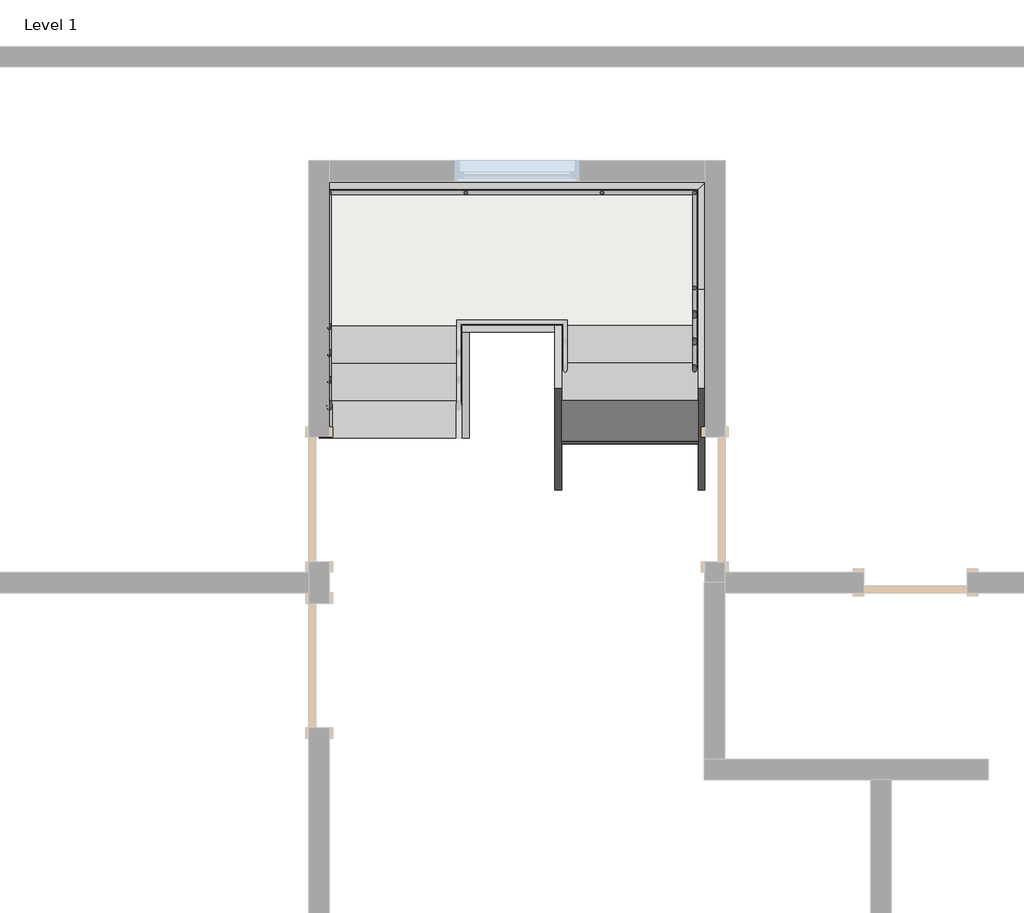
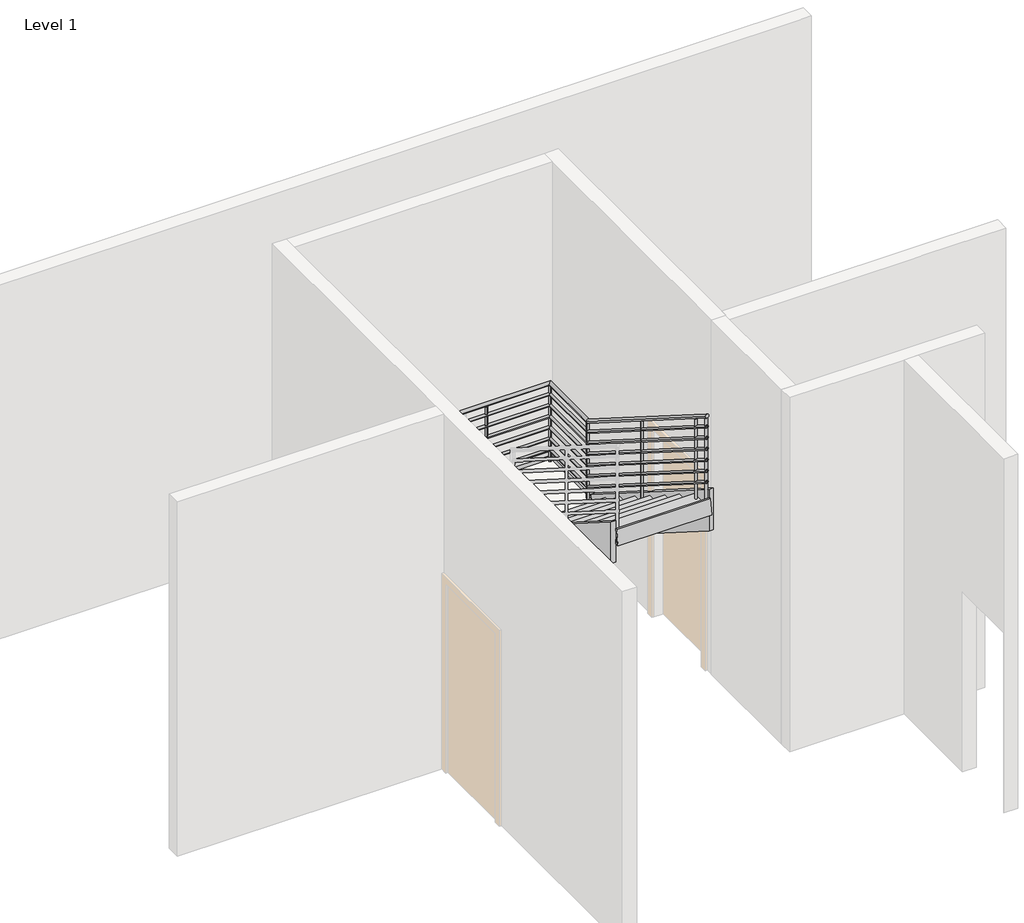
# One storey, part 3 of 3: 8 members, 2 stair flights, 1 railing, 1 slab.
"""IFC4 building model written with IfcOpenShell, lengths in millimetres."""

from ifc_helpers import new_model, si_unit, point, frame, frame_2d, origin, place, context, project, spatial, polyline, circle_curve, ellipse_curve, trimmed, segment, composite_curve, outline, extrude, faceted_brep, transform, mapped, element, save
from ifc_brep_helpers import plane_surface, cylinder_surface, advanced_brep
from components import non_monolithic_landing_4bf2fde8, stair_flight_50mm_tread_25mm_nosing_13mm_riser_7e2cbec3, stair_flight_50mm_tread_25mm_nosing_13mm_riser_d224a7c8

model = new_model("IFC4")

# Units and contexts
model_context = context("Model", 3, world=origin())
ifc_project = project(units=[si_unit("LENGTHUNIT", "METRE", prefix="MILLI")], contexts=[model_context])

# Site, building, storey
site = spatial("IfcSite", under=ifc_project)
building = spatial("IfcBuilding", under=site)
storey = spatial("IfcBuildingStorey", under=building, Name="Level 1", Elevation=0.0)

# Members
placement = place(None, origin())
element("IfcMember", 1, ObjectType="Stringer - 50mm Width", at=placement, inside=storey, context=model_context, shape_type="SweptSolid", body=[
    extrude(outline(polyline([(8997.57664, 0.0), (8997.57664, 215.089535), (9832.4076435, 743.0459009), (9948.2767035, 343.0459009), (9405.8353728, 0.0), (8997.57664, 0.0)])), frame((-10647.1504953, 0.0, 0.0), z_axis=(1.0, 0.0, 0.0), x_axis=(0.0, 1.0, 0.0)), (0.0, 0.0, 1.0), 50.0),
])
element("IfcMember", 2, ObjectType="Stringer - 50mm Width", at=placement, inside=storey, context=model_context, shape_type="SweptSolid", body=[
    extrude(outline(polyline([(8997.57664, 0.0), (8997.57664, 215.089535), (9772.57664, 705.2081121), (9772.57664, 231.9312362), (9405.8353728, 0.0), (8997.57664, 0.0)])), frame((-9597.1247141, 0.0, 0.0), z_axis=(1.0, 0.0, 0.0), x_axis=(0.0, 1.0, 0.0)), (0.0, 0.0, 1.0), 50.0),
])
element("IfcMember", 3, ObjectType="Stringer - 50mm Width", at=placement, inside=storey, context=model_context, shape_type="SweptSolid", body=[
    extrude(outline(polyline([(10087.7456364, 743.0459009), (9971.8765764, 343.0459009), (7897.57664, 1654.8561374), (7897.57664, 2128.1330133), (10087.7456364, 743.0459009)])), frame((-7867.4883818, 0.0, 0.0), z_axis=(1.0, 0.0, 0.0), x_axis=(0.0, 1.0, 0.0)), (0.0, 0.0, 1.0), 50.0),
])
element("IfcMember", 4, ObjectType="Stringer - 50mm Width", at=placement, inside=storey, context=model_context, shape_type="SweptSolid", body=[
    extrude(outline(polyline([(9822.57664, 910.7417089), (9822.57664, 437.464833), (7897.57664, 1654.8561374), (7897.57664, 2128.1330133), (9822.57664, 910.7417089)])), frame((-8917.5141631, 0.0, 0.0), z_axis=(1.0, 0.0, 0.0), x_axis=(0.0, 1.0, 0.0)), (0.0, 0.0, 1.0), 50.0),
])
element("IfcMember", 5, ObjectType="Stringer - 50mm Width", at=placement, inside=storey, context=model_context, shape_type="Brep", body=[
    faceted_brep([(-7867.4883818, 10087.7456364, 743.0459009), (-7817.4883818, 10087.7456364, 743.0459009), (-7817.4883818, 10872.6024212, 743.0459009), (-7867.4883818, 10822.6024212, 743.0459009), (-7867.4883818, 9971.8765764, 343.0459009), (-7867.4883818, 10822.6024212, 343.0459009), (-7817.4883818, 9971.8765764, 343.0459009), (-7817.4883818, 10872.6024212, 343.0459009)], [[[0, 1, 2, 3]], [[4, 0, 3, 5]], [[6, 4, 5, 7]], [[1, 6, 7, 2]], [[1, 0, 4, 6]], [[2, 7, 5, 3]]]),
])
element("IfcMember", 6, ObjectType="Stringer - 50mm Width", at=placement, inside=storey, context=model_context, shape_type="SweptSolid", body=[
    extrude(outline(polyline([(-7817.4883818, 10872.6024212), (-7867.4883818, 10822.6024212), (-10597.1504953, 10822.6024212), (-10647.1504953, 10872.6024212), (-7817.4883818, 10872.6024212)])), frame((0.0, 0.0, 343.0459009), z_axis=(0.0, 0.0, 1.0), x_axis=(1.0, 0.0, 0.0)), (0.0, 0.0, 1.0), 400.0),
])
element("IfcMember", 7, ObjectType="Stringer - 50mm Width", at=placement, inside=storey, context=model_context, shape_type="Brep", body=[
    faceted_brep([(-10597.1504953, 10822.6024212, 743.0459009), (-10647.1504953, 10872.6024212, 743.0459009), (-10647.1504953, 9832.4076435, 743.0459009), (-10597.1504953, 9832.4076435, 743.0459009), (-10597.1504953, 10822.6024212, 343.0459009), (-10597.1504953, 9948.2767035, 343.0459009), (-10647.1504953, 10872.6024212, 343.0459009), (-10647.1504953, 9948.2767035, 343.0459009)], [[[0, 1, 2, 3]], [[4, 0, 3, 5]], [[6, 4, 5, 7]], [[1, 6, 7, 2]], [[1, 0, 4, 6]], [[2, 7, 5, 3]]]),
])
element("IfcMember", 8, ObjectType="Stringer - 50mm Width", at=placement, inside=storey, context=model_context, shape_type="SweptSolid", body=[
    extrude(outline(polyline([(-9597.1247141, 9772.57664), (-9597.1247141, 9822.57664), (-8917.5141631, 9822.57664), (-8917.5141631, 9772.57664), (-9597.1247141, 9772.57664)])), frame((0.0, 0.0, 343.0459009), z_axis=(0.0, 0.0, 1.0), x_axis=(1.0, 0.0, 0.0)), (0.0, 0.0, 1.0), 400.0),
])

# Railing
element("IfcRailing", 9, ObjectType="900mm Pipe", at=placement, inside=storey, context=model_context, shape_type="SolidModel", body=[
    advanced_brep(
    [(-10551.7504953, 8997.57664, 1050.2491997), (-10591.7504953, 8997.57664, 1050.2491997), (-10551.7504953, 9828.370093, 1575.6521739), (-10591.7504953, 9828.370093, 1575.6521739), (-10551.7504953, 10777.2024212, 1575.6521739), (-10591.7504953, 10817.2024212, 1575.6521739), (-7912.8883818, 10777.2024212, 1575.6521739), (-7872.8883818, 10817.2024212, 1575.6521739), (-7912.8883818, 10091.783187, 1575.6521739), (-7872.8883818, 10091.783187, 1575.6521739), (-7912.8883818, 7897.57664, 2963.2926779), (-7872.8883818, 7897.57664, 2963.2926779)],
    [
        (0, 1, ellipse_curve(frame((-10571.7504953, 8997.57664, 1050.2491997), z_axis=(0.0, -1.0, 0.0), x_axis=(0.0, 0.0, -1.0)), 23.6638438, 20.0)),
        (1, 0, ellipse_curve(frame((-10571.7504953, 8997.57664, 1050.2491997), z_axis=(0.0, -1.0, 0.0), x_axis=(0.0, 0.0, -1.0)), 23.6638438, 20.0)),
        (0, 2),
        (2, 3, ellipse_curve(frame((-10571.7504953, 9828.370093, 1575.6521739), z_axis=(0.0, -0.9605132043335082, -0.27823440531497284), x_axis=(0.0, 0.2782344053149736, -0.9605132043335078)), 20.822202, 20.0)),
        (3, 1),
        (3, 2, ellipse_curve(frame((-10571.7504953, 9828.370093, 1575.6521739), z_axis=(0.0, -0.9605132043335082, -0.27823440531497284), x_axis=(0.0, 0.2782344053149736, -0.9605132043335078)), 20.822202, 20.0)),
        (2, 4),
        (4, 5, ellipse_curve(frame((-10571.7504953, 10797.2024212, 1575.6521739), z_axis=(-0.7071067811865475, -0.7071067811865475, 0.0), x_axis=(0.7071067811865474, -0.7071067811865476, 0.0)), 28.2842712, 20.0)),
        (5, 3),
        (5, 4, ellipse_curve(frame((-10571.7504953, 10797.2024212, 1575.6521739), z_axis=(-0.7071067811865475, -0.7071067811865475, 0.0), x_axis=(0.7071067811865474, -0.7071067811865476, 0.0)), 28.2842712, 20.0)),
        (4, 6),
        (6, 7, ellipse_curve(frame((-7892.8883818, 10797.2024212, 1575.6521739), z_axis=(-0.7071067811865475, 0.7071067811865475, 0.0), x_axis=(-0.7071067811865476, -0.7071067811865474, 0.0)), 28.2842712, 20.0)),
        (7, 5),
        (7, 6, ellipse_curve(frame((-7892.8883818, 10797.2024212, 1575.6521739), z_axis=(-0.7071067811865475, 0.7071067811865475, 0.0), x_axis=(-0.7071067811865476, -0.7071067811865474, 0.0)), 28.2842712, 20.0)),
        (6, 8),
        (8, 9, ellipse_curve(frame((-7892.8883818, 10091.783187, 1575.6521739), z_axis=(0.0, 0.9605132043335072, -0.27823440531497556), x_axis=(0.0, 0.27823440531497606, 0.9605132043335073)), 20.822202, 20.0)),
        (9, 7),
        (9, 8, ellipse_curve(frame((-7892.8883818, 10091.783187, 1575.6521739), z_axis=(0.0, 0.9605132043335072, -0.27823440531497556), x_axis=(0.0, 0.27823440531497606, 0.9605132043335073)), 20.822202, 20.0)),
        (10, 11, ellipse_curve(frame((-7892.8883818, 7897.57664, 2963.2926779), z_axis=(0.0, -1.0, 0.0), x_axis=(0.0, 0.0, -1.0)), 23.6638438, 20.0)),
        (11, 10, ellipse_curve(frame((-7892.8883818, 7897.57664, 2963.2926779), z_axis=(0.0, -1.0, 0.0), x_axis=(0.0, 0.0, -1.0)), 23.6638438, 20.0)),
        (8, 10),
        (11, 9),
    ],
    [
        plane_surface(frame((-10571.7504953, 8997.57664, 1073.9130435), z_axis=(0.0, -1.0, 0.0), x_axis=(0.0, 0.0, 1.0))),
        cylinder_surface(frame((-10571.7504953, 9008.2665528, 1057.0096189), z_axis=(0.0, -0.8451712313980468, -0.5344956404098252), x_axis=(-1.0, 0.0, 0.0)), 20.0),
        cylinder_surface(frame((-10571.7504953, 9822.57664, 1575.6521739), z_axis=(0.0, -1.0, 0.0), x_axis=(-1.0, 0.0, 0.0)), 20.0),
        cylinder_surface(frame((-10571.7504953, 10797.2024212, 1575.6521739), z_axis=(-1.0, 0.0, 0.0), x_axis=(0.0, 1.0, 0.0)), 20.0),
        cylinder_surface(frame((-7892.8883818, 10797.2024212, 1575.6521739), z_axis=(0.0, 1.0, 0.0), x_axis=(1.0, 0.0, 0.0)), 20.0),
        plane_surface(frame((-7892.8883818, 7897.57664, 2986.9565217), z_axis=(0.0, -1.0, 0.0), x_axis=(0.0, 0.0, -1.0))),
        cylinder_surface(frame((-7892.8883818, 10086.8867272, 1578.7487493), z_axis=(0.0, 0.8451712313980437, -0.5344956404098301), x_axis=(1.0, 0.0, 0.0)), 20.0),
    ],
    [
        (0, [[1, 2]]),
        (1, [[-1, 3, 4, 5]]),
        (1, [[-2, -5, 6, -3]]),
        (2, [[-4, 7, 8, 9]]),
        (2, [[-6, -9, 10, -7]]),
        (3, [[-8, 11, 12, 13]]),
        (3, [[-10, -13, 14, -11]]),
        (4, [[-12, 15, 16, 17]]),
        (4, [[-14, -17, 18, -15]]),
        (5, [[19, 20]]),
        (6, [[-16, 21, -20, 22]]),
        (6, [[-18, -22, -19, -21]]),
    ],
),
    advanced_brep(
    [(-10556.7504953, 8997.57664, 931.1651606), (-10586.7504953, 8997.57664, 931.1651606), (-10556.7504953, 9826.9217297, 1455.6521739), (-10586.7504953, 9826.9217297, 1455.6521739), (-10556.7504953, 10782.2024212, 1455.6521739), (-10586.7504953, 10812.2024212, 1455.6521739), (-7907.8883818, 10782.2024212, 1455.6521739), (-7877.8883818, 10812.2024212, 1455.6521739), (-7907.8883818, 10093.2315502, 1455.6521739), (-7877.8883818, 10093.2315502, 1455.6521739), (-7907.8883818, 7897.57664, 2844.2086389), (-7877.8883818, 7897.57664, 2844.2086389)],
    [
        (0, 1, ellipse_curve(frame((-10571.7504953, 8997.57664, 931.1651606), z_axis=(0.0, -1.0, 0.0), x_axis=(0.0, 0.0, -1.0)), 17.7478828, 15.0)),
        (1, 0, ellipse_curve(frame((-10571.7504953, 8997.57664, 931.1651606), z_axis=(0.0, -1.0, 0.0), x_axis=(0.0, 0.0, -1.0)), 17.7478828, 15.0)),
        (0, 2),
        (2, 3, ellipse_curve(frame((-10571.7504953, 9826.9217297, 1455.6521739), z_axis=(0.0, -0.9605132043335081, -0.2782344053149726), x_axis=(0.0, 0.27823440531497207, -0.9605132043335083)), 15.6166515, 15.0)),
        (3, 1),
        (3, 2, ellipse_curve(frame((-10571.7504953, 9826.9217297, 1455.6521739), z_axis=(0.0, -0.9605132043335081, -0.2782344053149726), x_axis=(0.0, 0.27823440531497207, -0.9605132043335083)), 15.6166515, 15.0)),
        (2, 4),
        (4, 5, ellipse_curve(frame((-10571.7504953, 10797.2024212, 1455.6521739), z_axis=(-0.7071067811865475, -0.7071067811865475, 0.0), x_axis=(0.7071067811865474, -0.7071067811865476, 0.0)), 21.2132034, 15.0)),
        (5, 3),
        (5, 4, ellipse_curve(frame((-10571.7504953, 10797.2024212, 1455.6521739), z_axis=(-0.7071067811865475, -0.7071067811865475, 0.0), x_axis=(0.7071067811865474, -0.7071067811865476, 0.0)), 21.2132034, 15.0)),
        (4, 6),
        (6, 7, ellipse_curve(frame((-7892.8883818, 10797.2024212, 1455.6521739), z_axis=(-0.7071067811865475, 0.7071067811865475, 0.0), x_axis=(-0.7071067811865476, -0.7071067811865474, 0.0)), 21.2132034, 15.0)),
        (7, 5),
        (7, 6, ellipse_curve(frame((-7892.8883818, 10797.2024212, 1455.6521739), z_axis=(-0.7071067811865475, 0.7071067811865475, 0.0), x_axis=(-0.7071067811865476, -0.7071067811865474, 0.0)), 21.2132034, 15.0)),
        (6, 8),
        (8, 9, ellipse_curve(frame((-7892.8883818, 10093.2315502, 1455.6521739), z_axis=(0.0, 0.9605132043335073, -0.27823440531497573), x_axis=(0.0, 0.27823440531497545, 0.9605132043335072)), 15.6166515, 15.0)),
        (9, 7),
        (9, 8, ellipse_curve(frame((-7892.8883818, 10093.2315502, 1455.6521739), z_axis=(0.0, 0.9605132043335073, -0.27823440531497573), x_axis=(0.0, 0.27823440531497545, 0.9605132043335072)), 15.6166515, 15.0)),
        (10, 11, ellipse_curve(frame((-7892.8883818, 7897.57664, 2844.2086389), z_axis=(0.0, -1.0, 0.0), x_axis=(0.0, 0.0, -1.0)), 17.7478828, 15.0)),
        (11, 10, ellipse_curve(frame((-7892.8883818, 7897.57664, 2844.2086389), z_axis=(0.0, -1.0, 0.0), x_axis=(0.0, 0.0, -1.0)), 17.7478828, 15.0)),
        (8, 10),
        (11, 9),
    ],
    [
        plane_surface(frame((-10571.7504953, 8997.57664, 948.9130435), z_axis=(0.0, -1.0, 0.0), x_axis=(0.0, 0.0, 1.0))),
        cylinder_surface(frame((-10571.7504953, 9005.5940746, 936.235475), z_axis=(0.0, -0.845171231398047, -0.534495640409825), x_axis=(-1.0, 0.0, 0.0)), 15.0),
        cylinder_surface(frame((-10571.7504953, 9822.57664, 1455.6521739), z_axis=(0.0, -1.0, 0.0), x_axis=(-1.0, 0.0, 0.0)), 15.0),
        cylinder_surface(frame((-10571.7504953, 10797.2024212, 1455.6521739), z_axis=(-1.0, 0.0, 0.0), x_axis=(0.0, 1.0, 0.0)), 15.0),
        cylinder_surface(frame((-7892.8883818, 10797.2024212, 1455.6521739), z_axis=(0.0, 1.0, 0.0), x_axis=(1.0, 0.0, 0.0)), 15.0),
        plane_surface(frame((-7892.8883818, 7897.57664, 2861.9565217), z_axis=(0.0, -1.0, 0.0), x_axis=(0.0, 0.0, -1.0))),
        cylinder_surface(frame((-7892.8883818, 10089.5592054, 1457.9746054), z_axis=(0.0, 0.8451712313980436, -0.5344956404098303), x_axis=(1.0, 0.0, 0.0)), 15.0),
    ],
    [
        (0, [[1, 2]]),
        (1, [[-1, 3, 4, 5]]),
        (1, [[-2, -5, 6, -3]]),
        (2, [[-4, 7, 8, 9]]),
        (2, [[-6, -9, 10, -7]]),
        (3, [[-8, 11, 12, 13]]),
        (3, [[-10, -13, 14, -11]]),
        (4, [[-12, 15, 16, 17]]),
        (4, [[-14, -17, 18, -15]]),
        (5, [[19, 20]]),
        (6, [[-16, 21, -20, 22]]),
        (6, [[-18, -22, -19, -21]]),
    ],
),
    advanced_brep(
    [(-10556.7504953, 8997.57664, 806.1651606), (-10586.7504953, 8997.57664, 806.1651606), (-10556.7504953, 9826.9217297, 1330.6521739), (-10586.7504953, 9826.9217297, 1330.6521739), (-10556.7504953, 10782.2024212, 1330.6521739), (-10586.7504953, 10812.2024212, 1330.6521739), (-7907.8883818, 10782.2024212, 1330.6521739), (-7877.8883818, 10812.2024212, 1330.6521739), (-7907.8883818, 10093.2315502, 1330.6521739), (-7877.8883818, 10093.2315502, 1330.6521739), (-7907.8883818, 7897.57664, 2719.2086389), (-7877.8883818, 7897.57664, 2719.2086389)],
    [
        (0, 1, ellipse_curve(frame((-10571.7504953, 8997.57664, 806.1651606), z_axis=(0.0, -1.0, 0.0), x_axis=(0.0, 0.0, -1.0)), 17.7478828, 15.0)),
        (1, 0, ellipse_curve(frame((-10571.7504953, 8997.57664, 806.1651606), z_axis=(0.0, -1.0, 0.0), x_axis=(0.0, 0.0, -1.0)), 17.7478828, 15.0)),
        (0, 2),
        (2, 3, ellipse_curve(frame((-10571.7504953, 9826.9217297, 1330.6521739), z_axis=(0.0, -0.9605132043335081, -0.2782344053149726), x_axis=(0.0, 0.27823440531497207, -0.9605132043335083)), 15.6166515, 15.0)),
        (3, 1),
        (3, 2, ellipse_curve(frame((-10571.7504953, 9826.9217297, 1330.6521739), z_axis=(0.0, -0.9605132043335081, -0.2782344053149726), x_axis=(0.0, 0.27823440531497207, -0.9605132043335083)), 15.6166515, 15.0)),
        (2, 4),
        (4, 5, ellipse_curve(frame((-10571.7504953, 10797.2024212, 1330.6521739), z_axis=(-0.7071067811865475, -0.7071067811865475, 0.0), x_axis=(0.7071067811865474, -0.7071067811865476, 0.0)), 21.2132034, 15.0)),
        (5, 3),
        (5, 4, ellipse_curve(frame((-10571.7504953, 10797.2024212, 1330.6521739), z_axis=(-0.7071067811865475, -0.7071067811865475, 0.0), x_axis=(0.7071067811865474, -0.7071067811865476, 0.0)), 21.2132034, 15.0)),
        (4, 6),
        (6, 7, ellipse_curve(frame((-7892.8883818, 10797.2024212, 1330.6521739), z_axis=(-0.7071067811865475, 0.7071067811865475, 0.0), x_axis=(-0.7071067811865476, -0.7071067811865474, 0.0)), 21.2132034, 15.0)),
        (7, 5),
        (7, 6, ellipse_curve(frame((-7892.8883818, 10797.2024212, 1330.6521739), z_axis=(-0.7071067811865475, 0.7071067811865475, 0.0), x_axis=(-0.7071067811865476, -0.7071067811865474, 0.0)), 21.2132034, 15.0)),
        (6, 8),
        (8, 9, ellipse_curve(frame((-7892.8883818, 10093.2315502, 1330.6521739), z_axis=(0.0, 0.9605132043335072, -0.2782344053149755), x_axis=(0.0, 0.27823440531497606, 0.9605132043335073)), 15.6166515, 15.0)),
        (9, 7),
        (9, 8, ellipse_curve(frame((-7892.8883818, 10093.2315502, 1330.6521739), z_axis=(0.0, 0.9605132043335072, -0.2782344053149755), x_axis=(0.0, 0.27823440531497606, 0.9605132043335073)), 15.6166515, 15.0)),
        (10, 11, ellipse_curve(frame((-7892.8883818, 7897.57664, 2719.2086389), z_axis=(0.0, -1.0, 0.0), x_axis=(0.0, 0.0, -1.0)), 17.7478828, 15.0)),
        (11, 10, ellipse_curve(frame((-7892.8883818, 7897.57664, 2719.2086389), z_axis=(0.0, -1.0, 0.0), x_axis=(0.0, 0.0, -1.0)), 17.7478828, 15.0)),
        (8, 10),
        (11, 9),
    ],
    [
        plane_surface(frame((-10571.7504953, 8997.57664, 823.9130435), z_axis=(0.0, -1.0, 0.0), x_axis=(0.0, 0.0, 1.0))),
        cylinder_surface(frame((-10571.7504953, 9005.5940746, 811.235475), z_axis=(0.0, -0.845171231398047, -0.534495640409825), x_axis=(-1.0, 0.0, 0.0)), 15.0),
        cylinder_surface(frame((-10571.7504953, 9822.57664, 1330.6521739), z_axis=(0.0, -1.0, 0.0), x_axis=(-1.0, 0.0, 0.0)), 15.0),
        cylinder_surface(frame((-10571.7504953, 10797.2024212, 1330.6521739), z_axis=(-1.0, 0.0, 0.0), x_axis=(0.0, 1.0, 0.0)), 15.0),
        cylinder_surface(frame((-7892.8883818, 10797.2024212, 1330.6521739), z_axis=(0.0, 1.0, 0.0), x_axis=(1.0, 0.0, 0.0)), 15.0),
        plane_surface(frame((-7892.8883818, 7897.57664, 2736.9565217), z_axis=(0.0, -1.0, 0.0), x_axis=(0.0, 0.0, -1.0))),
        cylinder_surface(frame((-7892.8883818, 10089.5592054, 1332.9746054), z_axis=(0.0, 0.8451712313980437, -0.5344956404098301), x_axis=(1.0, 0.0, 0.0)), 15.0),
    ],
    [
        (0, [[1, 2]]),
        (1, [[-1, 3, 4, 5]]),
        (1, [[-2, -5, 6, -3]]),
        (2, [[-4, 7, 8, 9]]),
        (2, [[-6, -9, 10, -7]]),
        (3, [[-8, 11, 12, 13]]),
        (3, [[-10, -13, 14, -11]]),
        (4, [[-12, 15, 16, 17]]),
        (4, [[-14, -17, 18, -15]]),
        (5, [[19, 20]]),
        (6, [[-16, 21, -20, 22]]),
        (6, [[-18, -22, -19, -21]]),
    ],
),
    advanced_brep(
    [(-10556.7504953, 8997.57664, 681.1651606), (-10586.7504953, 8997.57664, 681.1651606), (-10556.7504953, 9826.9217297, 1205.6521739), (-10586.7504953, 9826.9217297, 1205.6521739), (-10556.7504953, 10782.2024212, 1205.6521739), (-10586.7504953, 10812.2024212, 1205.6521739), (-7907.8883818, 10782.2024212, 1205.6521739), (-7877.8883818, 10812.2024212, 1205.6521739), (-7907.8883818, 10093.2315502, 1205.6521739), (-7877.8883818, 10093.2315502, 1205.6521739), (-7907.8883818, 7897.57664, 2594.2086389), (-7877.8883818, 7897.57664, 2594.2086389)],
    [
        (0, 1, ellipse_curve(frame((-10571.7504953, 8997.57664, 681.1651606), z_axis=(0.0, -1.0, 0.0), x_axis=(0.0, 0.0, -1.0)), 17.7478828, 15.0)),
        (1, 0, ellipse_curve(frame((-10571.7504953, 8997.57664, 681.1651606), z_axis=(0.0, -1.0, 0.0), x_axis=(0.0, 0.0, -1.0)), 17.7478828, 15.0)),
        (0, 2),
        (2, 3, ellipse_curve(frame((-10571.7504953, 9826.9217297, 1205.6521739), z_axis=(0.0, -0.9605132043335081, -0.2782344053149726), x_axis=(0.0, 0.27823440531497207, -0.9605132043335083)), 15.6166515, 15.0)),
        (3, 1),
        (3, 2, ellipse_curve(frame((-10571.7504953, 9826.9217297, 1205.6521739), z_axis=(0.0, -0.9605132043335081, -0.2782344053149726), x_axis=(0.0, 0.27823440531497207, -0.9605132043335083)), 15.6166515, 15.0)),
        (2, 4),
        (4, 5, ellipse_curve(frame((-10571.7504953, 10797.2024212, 1205.6521739), z_axis=(-0.7071067811865475, -0.7071067811865475, 0.0), x_axis=(0.7071067811865474, -0.7071067811865476, 0.0)), 21.2132034, 15.0)),
        (5, 3),
        (5, 4, ellipse_curve(frame((-10571.7504953, 10797.2024212, 1205.6521739), z_axis=(-0.7071067811865475, -0.7071067811865475, 0.0), x_axis=(0.7071067811865474, -0.7071067811865476, 0.0)), 21.2132034, 15.0)),
        (4, 6),
        (6, 7, ellipse_curve(frame((-7892.8883818, 10797.2024212, 1205.6521739), z_axis=(-0.7071067811865475, 0.7071067811865475, 0.0), x_axis=(-0.7071067811865476, -0.7071067811865474, 0.0)), 21.2132034, 15.0)),
        (7, 5),
        (7, 6, ellipse_curve(frame((-7892.8883818, 10797.2024212, 1205.6521739), z_axis=(-0.7071067811865475, 0.7071067811865475, 0.0), x_axis=(-0.7071067811865476, -0.7071067811865474, 0.0)), 21.2132034, 15.0)),
        (6, 8),
        (8, 9, ellipse_curve(frame((-7892.8883818, 10093.2315502, 1205.6521739), z_axis=(0.0, 0.9605132043335072, -0.2782344053149755), x_axis=(0.0, 0.27823440531497606, 0.9605132043335073)), 15.6166515, 15.0)),
        (9, 7),
        (9, 8, ellipse_curve(frame((-7892.8883818, 10093.2315502, 1205.6521739), z_axis=(0.0, 0.9605132043335072, -0.2782344053149755), x_axis=(0.0, 0.27823440531497606, 0.9605132043335073)), 15.6166515, 15.0)),
        (10, 11, ellipse_curve(frame((-7892.8883818, 7897.57664, 2594.2086389), z_axis=(0.0, -1.0, 0.0), x_axis=(0.0, 0.0, -1.0)), 17.7478828, 15.0)),
        (11, 10, ellipse_curve(frame((-7892.8883818, 7897.57664, 2594.2086389), z_axis=(0.0, -1.0, 0.0), x_axis=(0.0, 0.0, -1.0)), 17.7478828, 15.0)),
        (8, 10),
        (11, 9),
    ],
    [
        plane_surface(frame((-10571.7504953, 8997.57664, 698.9130435), z_axis=(0.0, -1.0, 0.0), x_axis=(0.0, 0.0, 1.0))),
        cylinder_surface(frame((-10571.7504953, 9005.5940746, 686.235475), z_axis=(0.0, -0.845171231398047, -0.534495640409825), x_axis=(-1.0, 0.0, 0.0)), 15.0),
        cylinder_surface(frame((-10571.7504953, 9822.57664, 1205.6521739), z_axis=(0.0, -1.0, 0.0), x_axis=(-1.0, 0.0, 0.0)), 15.0),
        cylinder_surface(frame((-10571.7504953, 10797.2024212, 1205.6521739), z_axis=(-1.0, 0.0, 0.0), x_axis=(0.0, 1.0, 0.0)), 15.0),
        cylinder_surface(frame((-7892.8883818, 10797.2024212, 1205.6521739), z_axis=(0.0, 1.0, 0.0), x_axis=(1.0, 0.0, 0.0)), 15.0),
        plane_surface(frame((-7892.8883818, 7897.57664, 2611.9565217), z_axis=(0.0, -1.0, 0.0), x_axis=(0.0, 0.0, -1.0))),
        cylinder_surface(frame((-7892.8883818, 10089.5592054, 1207.9746054), z_axis=(0.0, 0.8451712313980437, -0.5344956404098301), x_axis=(1.0, 0.0, 0.0)), 15.0),
    ],
    [
        (0, [[1, 2]]),
        (1, [[-1, 3, 4, 5]]),
        (1, [[-2, -5, 6, -3]]),
        (2, [[-4, 7, 8, 9]]),
        (2, [[-6, -9, 10, -7]]),
        (3, [[-8, 11, 12, 13]]),
        (3, [[-10, -13, 14, -11]]),
        (4, [[-12, 15, 16, 17]]),
        (4, [[-14, -17, 18, -15]]),
        (5, [[19, 20]]),
        (6, [[-16, 21, -20, 22]]),
        (6, [[-18, -22, -19, -21]]),
    ],
),
    advanced_brep(
    [(-10556.7504953, 8997.57664, 556.1651606), (-10586.7504953, 8997.57664, 556.1651606), (-10556.7504953, 9826.9217297, 1080.6521739), (-10586.7504953, 9826.9217297, 1080.6521739), (-10556.7504953, 10782.2024212, 1080.6521739), (-10586.7504953, 10812.2024212, 1080.6521739), (-7907.8883818, 10782.2024212, 1080.6521739), (-7877.8883818, 10812.2024212, 1080.6521739), (-7907.8883818, 10093.2315502, 1080.6521739), (-7877.8883818, 10093.2315502, 1080.6521739), (-7907.8883818, 7897.57664, 2469.2086389), (-7877.8883818, 7897.57664, 2469.2086389)],
    [
        (0, 1, ellipse_curve(frame((-10571.7504953, 8997.57664, 556.1651606), z_axis=(0.0, -1.0, 0.0), x_axis=(0.0, 0.0, -1.0)), 17.7478828, 15.0)),
        (1, 0, ellipse_curve(frame((-10571.7504953, 8997.57664, 556.1651606), z_axis=(0.0, -1.0, 0.0), x_axis=(0.0, 0.0, -1.0)), 17.7478828, 15.0)),
        (0, 2),
        (2, 3, ellipse_curve(frame((-10571.7504953, 9826.9217297, 1080.6521739), z_axis=(0.0, -0.9605132043335081, -0.27823440531497273), x_axis=(0.0, 0.2782344053149724, -0.9605132043335081)), 15.6166515, 15.0)),
        (3, 1),
        (3, 2, ellipse_curve(frame((-10571.7504953, 9826.9217297, 1080.6521739), z_axis=(0.0, -0.9605132043335081, -0.27823440531497273), x_axis=(0.0, 0.2782344053149724, -0.9605132043335081)), 15.6166515, 15.0)),
        (2, 4),
        (4, 5, ellipse_curve(frame((-10571.7504953, 10797.2024212, 1080.6521739), z_axis=(-0.7071067811865475, -0.7071067811865475, 0.0), x_axis=(0.7071067811865474, -0.7071067811865476, 0.0)), 21.2132034, 15.0)),
        (5, 3),
        (5, 4, ellipse_curve(frame((-10571.7504953, 10797.2024212, 1080.6521739), z_axis=(-0.7071067811865475, -0.7071067811865475, 0.0), x_axis=(0.7071067811865474, -0.7071067811865476, 0.0)), 21.2132034, 15.0)),
        (4, 6),
        (6, 7, ellipse_curve(frame((-7892.8883818, 10797.2024212, 1080.6521739), z_axis=(-0.7071067811865475, 0.7071067811865475, 0.0), x_axis=(-0.7071067811865476, -0.7071067811865474, 0.0)), 21.2132034, 15.0)),
        (7, 5),
        (7, 6, ellipse_curve(frame((-7892.8883818, 10797.2024212, 1080.6521739), z_axis=(-0.7071067811865475, 0.7071067811865475, 0.0), x_axis=(-0.7071067811865476, -0.7071067811865474, 0.0)), 21.2132034, 15.0)),
        (6, 8),
        (8, 9, ellipse_curve(frame((-7892.8883818, 10093.2315502, 1080.6521739), z_axis=(0.0, 0.9605132043335072, -0.2782344053149755), x_axis=(0.0, 0.27823440531497606, 0.9605132043335073)), 15.6166515, 15.0)),
        (9, 7),
        (9, 8, ellipse_curve(frame((-7892.8883818, 10093.2315502, 1080.6521739), z_axis=(0.0, 0.9605132043335072, -0.2782344053149755), x_axis=(0.0, 0.27823440531497606, 0.9605132043335073)), 15.6166515, 15.0)),
        (10, 11, ellipse_curve(frame((-7892.8883818, 7897.57664, 2469.2086389), z_axis=(0.0, -1.0, 0.0), x_axis=(0.0, 0.0, -1.0)), 17.7478828, 15.0)),
        (11, 10, ellipse_curve(frame((-7892.8883818, 7897.57664, 2469.2086389), z_axis=(0.0, -1.0, 0.0), x_axis=(0.0, 0.0, -1.0)), 17.7478828, 15.0)),
        (8, 10),
        (11, 9),
    ],
    [
        plane_surface(frame((-10571.7504953, 8997.57664, 573.9130435), z_axis=(0.0, -1.0, 0.0), x_axis=(0.0, 0.0, 1.0))),
        cylinder_surface(frame((-10571.7504953, 9005.5940746, 561.235475), z_axis=(0.0, -0.845171231398047, -0.5344956404098251), x_axis=(-1.0, 0.0, 0.0)), 15.0),
        cylinder_surface(frame((-10571.7504953, 9822.57664, 1080.6521739), z_axis=(0.0, -1.0, 0.0), x_axis=(-1.0, 0.0, 0.0)), 15.0),
        cylinder_surface(frame((-10571.7504953, 10797.2024212, 1080.6521739), z_axis=(-1.0, 0.0, 0.0), x_axis=(0.0, 1.0, 0.0)), 15.0),
        cylinder_surface(frame((-7892.8883818, 10797.2024212, 1080.6521739), z_axis=(0.0, 1.0, 0.0), x_axis=(1.0, 0.0, 0.0)), 15.0),
        plane_surface(frame((-7892.8883818, 7897.57664, 2486.9565217), z_axis=(0.0, -1.0, 0.0), x_axis=(0.0, 0.0, -1.0))),
        cylinder_surface(frame((-7892.8883818, 10089.5592054, 1082.9746054), z_axis=(0.0, 0.8451712313980437, -0.5344956404098301), x_axis=(1.0, 0.0, 0.0)), 15.0),
    ],
    [
        (0, [[1, 2]]),
        (1, [[-1, 3, 4, 5]]),
        (1, [[-2, -5, 6, -3]]),
        (2, [[-4, 7, 8, 9]]),
        (2, [[-6, -9, 10, -7]]),
        (3, [[-8, 11, 12, 13]]),
        (3, [[-10, -13, 14, -11]]),
        (4, [[-12, 15, 16, 17]]),
        (4, [[-14, -17, 18, -15]]),
        (5, [[19, 20]]),
        (6, [[-16, 21, -20, 22]]),
        (6, [[-18, -22, -19, -21]]),
    ],
),
    advanced_brep(
    [(-10556.7504953, 8997.57664, 431.1651606), (-10586.7504953, 8997.57664, 431.1651606), (-10556.7504953, 9826.9217297, 955.6521739), (-10586.7504953, 9826.9217297, 955.6521739), (-10556.7504953, 10782.2024212, 955.6521739), (-10586.7504953, 10812.2024212, 955.6521739), (-7907.8883818, 10782.2024212, 955.6521739), (-7877.8883818, 10812.2024212, 955.6521739), (-7907.8883818, 10093.2315502, 955.6521739), (-7877.8883818, 10093.2315502, 955.6521739), (-7907.8883818, 7897.57664, 2344.2086389), (-7877.8883818, 7897.57664, 2344.2086389)],
    [
        (0, 1, ellipse_curve(frame((-10571.7504953, 8997.57664, 431.1651606), z_axis=(0.0, -1.0, 0.0), x_axis=(0.0, 0.0, -1.0)), 17.7478828, 15.0)),
        (1, 0, ellipse_curve(frame((-10571.7504953, 8997.57664, 431.1651606), z_axis=(0.0, -1.0, 0.0), x_axis=(0.0, 0.0, -1.0)), 17.7478828, 15.0)),
        (0, 2),
        (2, 3, ellipse_curve(frame((-10571.7504953, 9826.9217297, 955.6521739), z_axis=(0.0, -0.9605132043335081, -0.27823440531497273), x_axis=(0.0, 0.2782344053149724, -0.9605132043335081)), 15.6166515, 15.0)),
        (3, 1),
        (3, 2, ellipse_curve(frame((-10571.7504953, 9826.9217297, 955.6521739), z_axis=(0.0, -0.9605132043335081, -0.27823440531497273), x_axis=(0.0, 0.2782344053149724, -0.9605132043335081)), 15.6166515, 15.0)),
        (2, 4),
        (4, 5, ellipse_curve(frame((-10571.7504953, 10797.2024212, 955.6521739), z_axis=(-0.7071067811865475, -0.7071067811865475, 0.0), x_axis=(0.7071067811865474, -0.7071067811865476, 0.0)), 21.2132034, 15.0)),
        (5, 3),
        (5, 4, ellipse_curve(frame((-10571.7504953, 10797.2024212, 955.6521739), z_axis=(-0.7071067811865475, -0.7071067811865475, 0.0), x_axis=(0.7071067811865474, -0.7071067811865476, 0.0)), 21.2132034, 15.0)),
        (4, 6),
        (6, 7, ellipse_curve(frame((-7892.8883818, 10797.2024212, 955.6521739), z_axis=(-0.7071067811865475, 0.7071067811865475, 0.0), x_axis=(-0.7071067811865476, -0.7071067811865474, 0.0)), 21.2132034, 15.0)),
        (7, 5),
        (7, 6, ellipse_curve(frame((-7892.8883818, 10797.2024212, 955.6521739), z_axis=(-0.7071067811865475, 0.7071067811865475, 0.0), x_axis=(-0.7071067811865476, -0.7071067811865474, 0.0)), 21.2132034, 15.0)),
        (6, 8),
        (8, 9, ellipse_curve(frame((-7892.8883818, 10093.2315502, 955.6521739), z_axis=(0.0, 0.9605132043335072, -0.2782344053149755), x_axis=(0.0, 0.27823440531497606, 0.9605132043335073)), 15.6166515, 15.0)),
        (9, 7),
        (9, 8, ellipse_curve(frame((-7892.8883818, 10093.2315502, 955.6521739), z_axis=(0.0, 0.9605132043335072, -0.2782344053149755), x_axis=(0.0, 0.27823440531497606, 0.9605132043335073)), 15.6166515, 15.0)),
        (10, 11, ellipse_curve(frame((-7892.8883818, 7897.57664, 2344.2086389), z_axis=(0.0, -1.0, 0.0), x_axis=(0.0, 0.0, -1.0)), 17.7478828, 15.0)),
        (11, 10, ellipse_curve(frame((-7892.8883818, 7897.57664, 2344.2086389), z_axis=(0.0, -1.0, 0.0), x_axis=(0.0, 0.0, -1.0)), 17.7478828, 15.0)),
        (8, 10),
        (11, 9),
    ],
    [
        plane_surface(frame((-10571.7504953, 8997.57664, 448.9130435), z_axis=(0.0, -1.0, 0.0), x_axis=(0.0, 0.0, 1.0))),
        cylinder_surface(frame((-10571.7504953, 9005.5940746, 436.235475), z_axis=(0.0, -0.845171231398047, -0.5344956404098251), x_axis=(-1.0, 0.0, 0.0)), 15.0),
        cylinder_surface(frame((-10571.7504953, 9822.57664, 955.6521739), z_axis=(0.0, -1.0, 0.0), x_axis=(-1.0, 0.0, 0.0)), 15.0),
        cylinder_surface(frame((-10571.7504953, 10797.2024212, 955.6521739), z_axis=(-1.0, 0.0, 0.0), x_axis=(0.0, 1.0, 0.0)), 15.0),
        cylinder_surface(frame((-7892.8883818, 10797.2024212, 955.6521739), z_axis=(0.0, 1.0, 0.0), x_axis=(1.0, 0.0, 0.0)), 15.0),
        plane_surface(frame((-7892.8883818, 7897.57664, 2361.9565217), z_axis=(0.0, -1.0, 0.0), x_axis=(0.0, 0.0, -1.0))),
        cylinder_surface(frame((-7892.8883818, 10089.5592054, 957.9746054), z_axis=(0.0, 0.8451712313980437, -0.5344956404098301), x_axis=(1.0, 0.0, 0.0)), 15.0),
    ],
    [
        (0, [[1, 2]]),
        (1, [[-1, 3, 4, 5]]),
        (1, [[-2, -5, 6, -3]]),
        (2, [[-4, 7, 8, 9]]),
        (2, [[-6, -9, 10, -7]]),
        (3, [[-8, 11, 12, 13]]),
        (3, [[-10, -13, 14, -11]]),
        (4, [[-12, 15, 16, 17]]),
        (4, [[-14, -17, 18, -15]]),
        (5, [[19, 20]]),
        (6, [[-16, 21, -20, 22]]),
        (6, [[-18, -22, -19, -21]]),
    ],
),
    advanced_brep(
    [(-10556.7504953, 8997.57664, 306.1651606), (-10586.7504953, 8997.57664, 306.1651606), (-10556.7504953, 9826.9217297, 830.6521739), (-10586.7504953, 9826.9217297, 830.6521739), (-10556.7504953, 10782.2024212, 830.6521739), (-10586.7504953, 10812.2024212, 830.6521739), (-7907.8883818, 10782.2024212, 830.6521739), (-7877.8883818, 10812.2024212, 830.6521739), (-7907.8883818, 10093.2315502, 830.6521739), (-7877.8883818, 10093.2315502, 830.6521739), (-7907.8883818, 7897.57664, 2219.2086389), (-7877.8883818, 7897.57664, 2219.2086389)],
    [
        (0, 1, ellipse_curve(frame((-10571.7504953, 8997.57664, 306.1651606), z_axis=(0.0, -1.0, 0.0), x_axis=(0.0, 0.0, -1.0)), 17.7478828, 15.0)),
        (1, 0, ellipse_curve(frame((-10571.7504953, 8997.57664, 306.1651606), z_axis=(0.0, -1.0, 0.0), x_axis=(0.0, 0.0, -1.0)), 17.7478828, 15.0)),
        (0, 2),
        (2, 3, ellipse_curve(frame((-10571.7504953, 9826.9217297, 830.6521739), z_axis=(0.0, -0.9605132043335081, -0.27823440531497273), x_axis=(0.0, 0.2782344053149724, -0.9605132043335081)), 15.6166515, 15.0)),
        (3, 1),
        (3, 2, ellipse_curve(frame((-10571.7504953, 9826.9217297, 830.6521739), z_axis=(0.0, -0.9605132043335081, -0.27823440531497273), x_axis=(0.0, 0.2782344053149724, -0.9605132043335081)), 15.6166515, 15.0)),
        (2, 4),
        (4, 5, ellipse_curve(frame((-10571.7504953, 10797.2024212, 830.6521739), z_axis=(-0.7071067811865475, -0.7071067811865475, 0.0), x_axis=(0.7071067811865474, -0.7071067811865476, 0.0)), 21.2132034, 15.0)),
        (5, 3),
        (5, 4, ellipse_curve(frame((-10571.7504953, 10797.2024212, 830.6521739), z_axis=(-0.7071067811865475, -0.7071067811865475, 0.0), x_axis=(0.7071067811865474, -0.7071067811865476, 0.0)), 21.2132034, 15.0)),
        (4, 6),
        (6, 7, ellipse_curve(frame((-7892.8883818, 10797.2024212, 830.6521739), z_axis=(-0.7071067811865475, 0.7071067811865475, 0.0), x_axis=(-0.7071067811865476, -0.7071067811865474, 0.0)), 21.2132034, 15.0)),
        (7, 5),
        (7, 6, ellipse_curve(frame((-7892.8883818, 10797.2024212, 830.6521739), z_axis=(-0.7071067811865475, 0.7071067811865475, 0.0), x_axis=(-0.7071067811865476, -0.7071067811865474, 0.0)), 21.2132034, 15.0)),
        (6, 8),
        (8, 9, ellipse_curve(frame((-7892.8883818, 10093.2315502, 830.6521739), z_axis=(0.0, 0.9605132043335072, -0.2782344053149755), x_axis=(0.0, 0.27823440531497606, 0.9605132043335073)), 15.6166515, 15.0)),
        (9, 7),
        (9, 8, ellipse_curve(frame((-7892.8883818, 10093.2315502, 830.6521739), z_axis=(0.0, 0.9605132043335072, -0.2782344053149755), x_axis=(0.0, 0.27823440531497606, 0.9605132043335073)), 15.6166515, 15.0)),
        (10, 11, ellipse_curve(frame((-7892.8883818, 7897.57664, 2219.2086389), z_axis=(0.0, -1.0, 0.0), x_axis=(0.0, 0.0, -1.0)), 17.7478828, 15.0)),
        (11, 10, ellipse_curve(frame((-7892.8883818, 7897.57664, 2219.2086389), z_axis=(0.0, -1.0, 0.0), x_axis=(0.0, 0.0, -1.0)), 17.7478828, 15.0)),
        (8, 10),
        (11, 9),
    ],
    [
        plane_surface(frame((-10571.7504953, 8997.57664, 323.9130435), z_axis=(0.0, -1.0, 0.0), x_axis=(0.0, 0.0, 1.0))),
        cylinder_surface(frame((-10571.7504953, 9005.5940746, 311.235475), z_axis=(0.0, -0.845171231398047, -0.5344956404098251), x_axis=(-1.0, 0.0, 0.0)), 15.0),
        cylinder_surface(frame((-10571.7504953, 9822.57664, 830.6521739), z_axis=(0.0, -1.0, 0.0), x_axis=(-1.0, 0.0, 0.0)), 15.0),
        cylinder_surface(frame((-10571.7504953, 10797.2024212, 830.6521739), z_axis=(-1.0, 0.0, 0.0), x_axis=(0.0, 1.0, 0.0)), 15.0),
        cylinder_surface(frame((-7892.8883818, 10797.2024212, 830.6521739), z_axis=(0.0, 1.0, 0.0), x_axis=(1.0, 0.0, 0.0)), 15.0),
        plane_surface(frame((-7892.8883818, 7897.57664, 2236.9565217), z_axis=(0.0, -1.0, 0.0), x_axis=(0.0, 0.0, -1.0))),
        cylinder_surface(frame((-7892.8883818, 10089.5592054, 832.9746054), z_axis=(0.0, 0.8451712313980437, -0.5344956404098301), x_axis=(1.0, 0.0, 0.0)), 15.0),
    ],
    [
        (0, [[1, 2]]),
        (1, [[-1, 3, 4, 5]]),
        (1, [[-2, -5, 6, -3]]),
        (2, [[-4, 7, 8, 9]]),
        (2, [[-6, -9, 10, -7]]),
        (3, [[-8, 11, 12, 13]]),
        (3, [[-10, -13, 14, -11]]),
        (4, [[-12, 15, 16, 17]]),
        (4, [[-14, -17, 18, -15]]),
        (5, [[19, 20]]),
        (6, [[-16, 21, -20, 22]]),
        (6, [[-18, -22, -19, -21]]),
    ],
),
    advanced_brep(
    [(-7880.3883818, 8097.57664, 2813.1466207), (-7905.3883818, 8097.57664, 2813.1466207), (-7905.3883818, 8097.57664, 1913.0434783), (-7880.3883818, 8097.57664, 1913.0434783)],
    [
        (0, 1, ellipse_curve(frame((-7892.8883818, 8097.57664, 2813.1466207), z_axis=(0.0, -0.5344956404098302, -0.8451712313980437), x_axis=(0.0, -0.8451712313980437, 0.53449564040983)), 14.7899024, 12.5)),
        (1, 2),
        (2, 3, circle_curve(frame((-7892.8883818, 8097.57664, 1913.0434783), z_axis=(0.0, 0.0, 1.0), x_axis=(-1.0, 0.0, 0.0)), 12.5)),
        (3, 0),
        (3, 2, circle_curve(frame((-7892.8883818, 8097.57664, 1913.0434783), z_axis=(0.0, 0.0, 1.0), x_axis=(-1.0, 0.0, 0.0)), 12.5)),
        (1, 0, ellipse_curve(frame((-7892.8883818, 8097.57664, 2813.1466207), z_axis=(0.0, -0.5344956404098302, -0.8451712313980437), x_axis=(0.0, -0.8451712313980437, 0.53449564040983)), 14.7899024, 12.5)),
    ],
    [
        cylinder_surface(frame((-7892.8883818, 8097.57664, 1813.0434783), z_axis=(0.0, 0.0, 1.0), x_axis=(-1.0, 0.0, 0.0)), 12.5),
        plane_surface(frame((-7917.8883818, 8072.57664, 2828.9568974), z_axis=(0.0, 0.5344956404098302, 0.8451712313980437), x_axis=(1.0, 0.0, 0.0))),
        plane_surface(frame((-7917.8883818, 8122.57664, 1913.0434783), z_axis=(0.0, 0.0, -1.0), x_axis=(1.0, 0.0, 0.0))),
    ],
    [
        (0, [[1, 2, 3, 4]]),
        (0, [[5, -2, 6, -4]]),
        (1, [[-6, -1]]),
        (2, [[-5, -3]]),
    ],
),
    advanced_brep(
    [(-7880.3883818, 9097.57664, 2180.7355535), (-7905.3883818, 9097.57664, 2180.7355535), (-7905.3883818, 9097.57664, 1217.3913043), (-7880.3883818, 9097.57664, 1217.3913043)],
    [
        (0, 1, ellipse_curve(frame((-7892.8883818, 9097.57664, 2180.7355535), z_axis=(0.0, -0.5344956404098302, -0.8451712313980437), x_axis=(0.0, -0.8451712313980437, 0.53449564040983)), 14.7899024, 12.5)),
        (1, 2),
        (2, 3, circle_curve(frame((-7892.8883818, 9097.57664, 1217.3913043), z_axis=(0.0, 0.0, 1.0), x_axis=(-1.0, 0.0, 0.0)), 12.5)),
        (3, 0),
        (3, 2, circle_curve(frame((-7892.8883818, 9097.57664, 1217.3913043), z_axis=(0.0, 0.0, 1.0), x_axis=(-1.0, 0.0, 0.0)), 12.5)),
        (1, 0, ellipse_curve(frame((-7892.8883818, 9097.57664, 2180.7355535), z_axis=(0.0, -0.5344956404098302, -0.8451712313980437), x_axis=(0.0, -0.8451712313980437, 0.53449564040983)), 14.7899024, 12.5)),
    ],
    [
        cylinder_surface(frame((-7892.8883818, 9097.57664, 1117.3913043), z_axis=(0.0, 0.0, 1.0), x_axis=(-1.0, 0.0, 0.0)), 12.5),
        plane_surface(frame((-7917.8883818, 9072.57664, 2196.5458302), z_axis=(0.0, 0.5344956404098302, 0.8451712313980437), x_axis=(1.0, 0.0, 0.0))),
        plane_surface(frame((-7917.8883818, 9122.57664, 1217.3913043), z_axis=(0.0, 0.0, -1.0), x_axis=(1.0, 0.0, 0.0))),
    ],
    [
        (0, [[1, 2, 3, 4]]),
        (0, [[5, -2, 6, -4]]),
        (1, [[-6, -1]]),
        (2, [[-5, -3]]),
    ],
),
    extrude(outline(composite_curve([segment(trimmed(circle_curve(frame_2d((-8571.7504953, 10797.2024212)), 12.5), [point((-8571.7504953, 10784.7024212))], [point((-8571.7504953, 10809.7024212))], False, "CARTESIAN"), True, "CONTINUOUS"), segment(trimmed(circle_curve(frame_2d((-8571.7504953, 10797.2024212)), 12.5), [point((-8571.7504953, 10809.7024212))], [point((-8571.7504953, 10784.7024212))], False, "CARTESIAN"), True, "CONTINUOUS")], self_intersect=False)), frame((0.0, 0.0, 695.6521739), z_axis=(0.0, 0.0, 1.0), x_axis=(1.0, 0.0, 0.0)), (0.0, 0.0, 1.0), 860.0),
    extrude(outline(composite_curve([segment(trimmed(circle_curve(frame_2d((-9571.7504953, 10797.2024212)), 12.5), [point((-9571.7504953, 10784.7024212))], [point((-9571.7504953, 10809.7024212))], False, "CARTESIAN"), True, "CONTINUOUS"), segment(trimmed(circle_curve(frame_2d((-9571.7504953, 10797.2024212)), 12.5), [point((-9571.7504953, 10809.7024212))], [point((-9571.7504953, 10784.7024212))], False, "CARTESIAN"), True, "CONTINUOUS")], self_intersect=False)), frame((0.0, 0.0, 695.6521739), z_axis=(0.0, 0.0, 1.0), x_axis=(1.0, 0.0, 0.0)), (0.0, 0.0, 1.0), 860.0),
    extrude(outline(composite_curve([segment(trimmed(circle_curve(frame_2d((-7892.8883818, 10097.57664)), 12.5), [point((-7905.3883818, 10097.57664))], [point((-7880.3883818, 10097.57664))], False, "CARTESIAN"), True, "CONTINUOUS"), segment(trimmed(circle_curve(frame_2d((-7892.8883818, 10097.57664)), 12.5), [point((-7880.3883818, 10097.57664))], [point((-7905.3883818, 10097.57664))], False, "CARTESIAN"), True, "CONTINUOUS")], self_intersect=False)), frame((0.0, 0.0, 695.6521739), z_axis=(0.0, 0.0, 1.0), x_axis=(1.0, 0.0, 0.0)), (0.0, 0.0, 1.0), 860.0),
    extrude(outline(composite_curve([segment(trimmed(circle_curve(frame_2d((-7892.8883818, 10797.2024212)), 12.5), [point((-7892.8883818, 10784.7024212))], [point((-7892.8883818, 10809.7024212))], False, "CARTESIAN"), True, "CONTINUOUS"), segment(trimmed(circle_curve(frame_2d((-7892.8883818, 10797.2024212)), 12.5), [point((-7892.8883818, 10809.7024212))], [point((-7892.8883818, 10784.7024212))], False, "CARTESIAN"), True, "CONTINUOUS")], self_intersect=False)), frame((0.0, 0.0, 695.6521739), z_axis=(0.0, 0.0, 1.0), x_axis=(1.0, 0.0, 0.0)), (0.0, 0.0, 1.0), 860.0),
    extrude(outline(composite_curve([segment(trimmed(circle_curve(frame_2d((-10571.7504953, 10797.2024212)), 12.5), [point((-10559.2504953, 10797.2024212))], [point((-10584.2504953, 10797.2024212))], False, "CARTESIAN"), True, "CONTINUOUS"), segment(trimmed(circle_curve(frame_2d((-10571.7504953, 10797.2024212)), 12.5), [point((-10584.2504953, 10797.2024212))], [point((-10559.2504953, 10797.2024212))], False, "CARTESIAN"), True, "CONTINUOUS")], self_intersect=False)), frame((0.0, 0.0, 695.6521739), z_axis=(0.0, 0.0, 1.0), x_axis=(1.0, 0.0, 0.0)), (0.0, 0.0, 1.0), 860.0),
    extrude(outline(composite_curve([segment(trimmed(circle_curve(frame_2d((-10571.7504953, 9822.57664)), 12.5), [point((-10559.2504953, 9822.57664))], [point((-10584.2504953, 9822.57664))], False, "CARTESIAN"), True, "CONTINUOUS"), segment(trimmed(circle_curve(frame_2d((-10571.7504953, 9822.57664)), 12.5), [point((-10584.2504953, 9822.57664))], [point((-10559.2504953, 9822.57664))], False, "CARTESIAN"), True, "CONTINUOUS")], self_intersect=False)), frame((0.0, 0.0, 695.6521739), z_axis=(0.0, 0.0, 1.0), x_axis=(1.0, 0.0, 0.0)), (0.0, 0.0, 1.0), 860.0),
    advanced_brep(
    [(-7880.3883818, 7910.07664, 2931.7236958), (-7905.3883818, 7910.07664, 2931.7236958), (-7905.3883818, 7910.07664, 1913.0434783), (-7880.3883818, 7910.07664, 1913.0434783)],
    [
        (0, 1, ellipse_curve(frame((-7892.8883818, 7910.07664, 2931.7236958), z_axis=(0.0, -0.5344956404098302, -0.8451712313980437), x_axis=(0.0, -0.8451712313980437, 0.53449564040983)), 14.7899024, 12.5)),
        (1, 2),
        (2, 3, circle_curve(frame((-7892.8883818, 7910.07664, 1913.0434783), z_axis=(0.0, 0.0, 1.0), x_axis=(-1.0, 0.0, 0.0)), 12.5)),
        (3, 0),
        (3, 2, circle_curve(frame((-7892.8883818, 7910.07664, 1913.0434783), z_axis=(0.0, 0.0, 1.0), x_axis=(-1.0, 0.0, 0.0)), 12.5)),
        (1, 0, ellipse_curve(frame((-7892.8883818, 7910.07664, 2931.7236958), z_axis=(0.0, -0.5344956404098302, -0.8451712313980437), x_axis=(0.0, -0.8451712313980437, 0.53449564040983)), 14.7899024, 12.5)),
    ],
    [
        cylinder_surface(frame((-7892.8883818, 7910.07664, 1813.0434783), z_axis=(0.0, 0.0, 1.0), x_axis=(-1.0, 0.0, 0.0)), 12.5),
        plane_surface(frame((-7917.8883818, 7885.07664, 2947.5339725), z_axis=(0.0, 0.5344956404098302, 0.8451712313980437), x_axis=(1.0, 0.0, 0.0))),
        plane_surface(frame((-7917.8883818, 7935.07664, 1913.0434783), z_axis=(0.0, 0.0, -1.0), x_axis=(1.0, 0.0, 0.0))),
    ],
    [
        (0, [[1, 2, 3, 4]]),
        (0, [[5, -2, 6, -4]]),
        (1, [[-6, -1]]),
        (2, [[-5, -3]]),
    ],
),
    advanced_brep(
    [(-10584.2504953, 9010.07664, 1034.4904942), (-10559.2504953, 9010.07664, 1034.4904942), (-10559.2504953, 9010.07664, 173.9130435), (-10584.2504953, 9010.07664, 173.9130435)],
    [
        (0, 1, ellipse_curve(frame((-10571.7504953, 9010.07664, 1034.4904942), z_axis=(0.0, 0.5344956404098368, -0.8451712313980396), x_axis=(0.0, 0.8451712313980398, 0.5344956404098364)), 14.7899024, 12.5)),
        (1, 2),
        (2, 3, circle_curve(frame((-10571.7504953, 9010.07664, 173.9130435), z_axis=(0.0, 0.0, 1.0), x_axis=(1.0, 0.0, 0.0)), 12.5)),
        (3, 0),
        (3, 2, circle_curve(frame((-10571.7504953, 9010.07664, 173.9130435), z_axis=(0.0, 0.0, 1.0), x_axis=(1.0, 0.0, 0.0)), 12.5)),
        (1, 0, ellipse_curve(frame((-10571.7504953, 9010.07664, 1034.4904942), z_axis=(0.0, 0.5344956404098368, -0.8451712313980396), x_axis=(0.0, 0.8451712313980398, 0.5344956404098364)), 14.7899024, 12.5)),
    ],
    [
        cylinder_surface(frame((-10571.7504953, 9010.07664, 73.9130435), z_axis=(0.0, 0.0, 1.0), x_axis=(1.0, 0.0, 0.0)), 12.5),
        plane_surface(frame((-10546.7504953, 9035.07664, 1050.3007709), z_axis=(0.0, -0.5344956404098368, 0.8451712313980396), x_axis=(-1.0, 0.0, 0.0))),
        plane_surface(frame((-10546.7504953, 8985.07664, 173.9130435), z_axis=(0.0, 0.0, -1.0), x_axis=(-1.0, 0.0, 0.0))),
    ],
    [
        (0, [[1, 2, 3, 4]]),
        (0, [[5, -2, 6, -4]]),
        (1, [[-6, -1]]),
        (2, [[-5, -3]]),
    ],
),
])

# Slab
non_monolithic_landing_shape = non_monolithic_landing_4bf2fde8(model_context)
element("IfcSlab", 10, ObjectType="Non-Monolithic Landing", at=placement, inside=storey, context=model_context, shape_type="MappedRepresentation", body=[
    mapped(non_monolithic_landing_shape, transform((0.0, 0.0, 0.0), x_axis=(1.0, 0.0, 0.0), y_axis=(0.0, 1.0, 0.0), z_axis=(0.0, 0.0, 1.0))),
])

# Stair flights
stair_flight_50mm_tread_25mm_nosing_13mm_riser_shape = stair_flight_50mm_tread_25mm_nosing_13mm_riser_7e2cbec3(model_context)
element("IfcStairFlight", 11, ObjectType="50mm Tread 25mm Nosing 13mm Riser", at=placement, inside=storey, context=model_context, shape_type="MappedRepresentation", body=[
    mapped(stair_flight_50mm_tread_25mm_nosing_13mm_riser_shape, transform((0.0, 0.0, 0.0), x_axis=(1.0, 0.0, 0.0), y_axis=(0.0, 1.0, 0.0), z_axis=(0.0, 0.0, 1.0))),
])
stair_flight_50mm_tread_25mm_nosing_13mm_riser_2_shape = stair_flight_50mm_tread_25mm_nosing_13mm_riser_d224a7c8(model_context)
element("IfcStairFlight", 12, ObjectType="50mm Tread 25mm Nosing 13mm Riser", at=placement, inside=storey, context=model_context, shape_type="MappedRepresentation", body=[
    mapped(stair_flight_50mm_tread_25mm_nosing_13mm_riser_2_shape, transform((0.0, 0.0, 0.0), x_axis=(1.0, 0.0, 0.0), y_axis=(0.0, 1.0, 0.0), z_axis=(0.0, 0.0, 1.0))),
])

save(model, "model.ifc")

# Revit data of these elements
# Type "900mm Pipe"
#   built-in parameter 1008612 = 0.019685 (stored number, unit not read)
#   built-in parameter 1008611 = 0.0984252 (stored number, unit not read)
#   built-in parameter 1008609 = 6.56168 (stored number, unit not read)
#   built-in parameter 1008604 = 0.19685 (stored number, unit not read)
#   built-in parameter 1008603 = 0.164042 (stored number, unit not read)
#   Railing Height = 900 mm
#   built-in parameter 1008630 = 2
#   built-in parameter 1008610 = 2
#   built-in parameter 1008605 = 1
#   built-in parameter 1008618 = M_Baluster - Round : 25mm
# Elements 1, 2, 3, 4, 5, 6, 7, 8 (IfcMember, "Stringer - 50mm Width")
#   Phase Created = New Construction
# Element 9 (IfcRailing, "900mm Pipe")
#   Phase Created = New Construction
# Element 10 (IfcSlab, "Non-Monolithic Landing")
#   Phase Created = New Construction
# Elements 11, 12 (IfcStairFlight, "50mm Tread 25mm Nosing 13mm Riser")
#   Phase Created = New Construction
